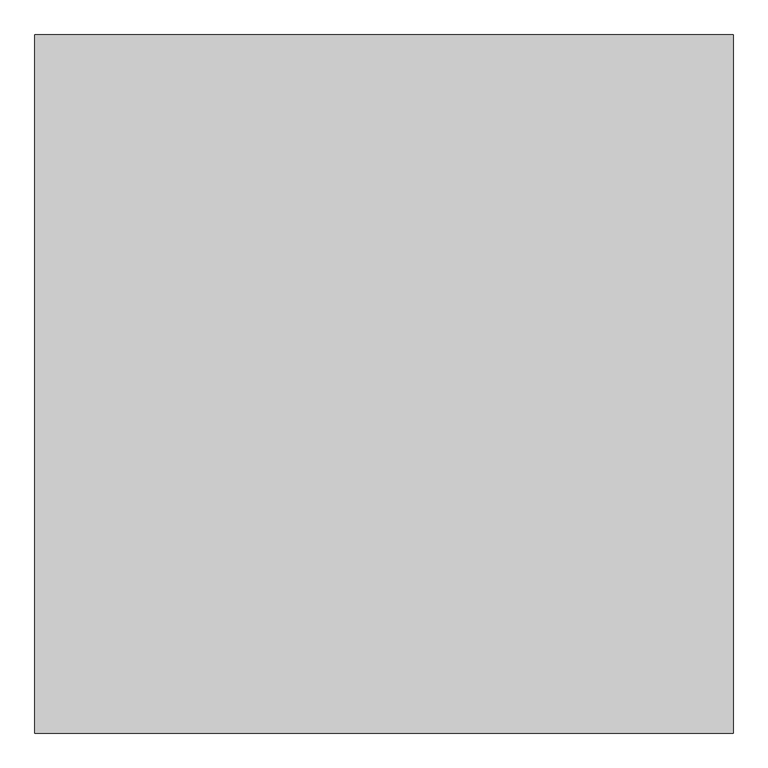
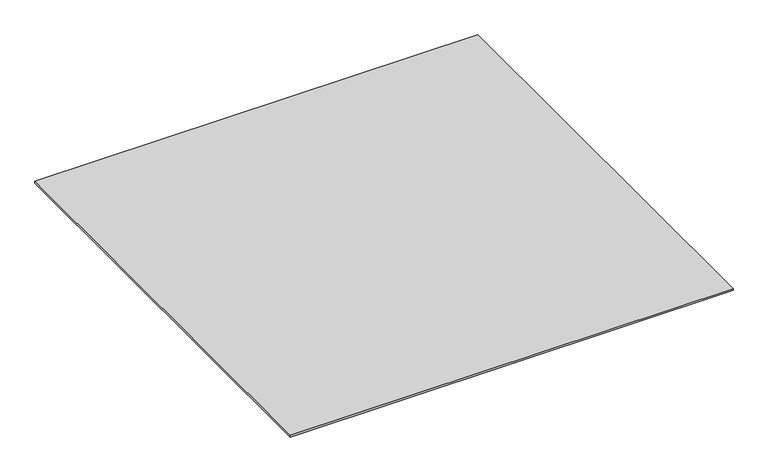
"""IFC4 building model written with IfcOpenShell, lengths in millimetres: furniture geometry."""

from ifc_helpers import new_model, si_unit, origin, origin_with_axes, place, context, project, spatial, polyline, outline, extrude, source, transform, mapped, element, save


def furniture_e65422ec(model_context):
    return source(origin(), model_context, "Body", "SweptSolid", [
        extrude(outline(polyline([(1250.0, -1250.0), (-1250.0, -1250.0), (-1250.0, 1250.0), (1250.0, 1250.0), (1250.0, -1250.0)])), origin_with_axes(), (0.0, 0.0, 1.0), 10.0),
    ])


if __name__ == "__main__":
    model = new_model("IFC4")
    model_context = context("Model", 3, world=origin())
    ifc_project = project(units=[si_unit("LENGTHUNIT", "METRE", prefix="MILLI")], contexts=[model_context])
    site = spatial("IfcSite", under=ifc_project)
    building = spatial("IfcBuilding", under=site)
    placement = place(None, origin())
    furniture_shape = furniture_e65422ec(model_context)
    element("IfcFurniture", 1, at=placement, inside=building, context=model_context, shape_type="MappedRepresentation", body=[
        mapped(furniture_shape, transform((0.0, 0.0, 0.0), x_axis=(1.0, 0.0, 0.0), y_axis=(0.0, 1.0, 0.0), z_axis=(0.0, 0.0, 1.0))),
    ])
    save(model, "model.ifc")

# Revit data of these elements
# Type
#   Width - Anchura = 2500 mm
#   Thickness - Espesor = 10 mm
#   Large - Largo = 2500 mm
#   Default Elevation = 1219.2 mm
